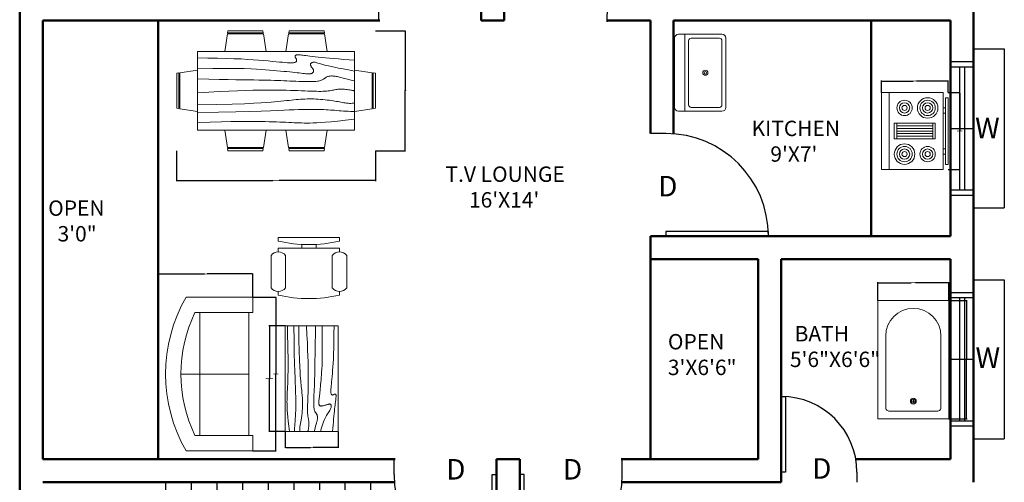
# Model space of a CAD drawing. Units: inches. Extents: x -8 to 1354, y -679 to 94.
# Tile 2 of 6: x 4 to 388, y -429 to -248. Entities that reach past the tile are written whole.
import ezdxf

# ---------------------------------------------------------------- set-up
doc = ezdxf.new("R2010")
doc.units = ezdxf.units.IN
doc.header["$MEASUREMENT"] = 0
for name, color, linetype, lineweight in [('A-ANNO-DIMS', 2, 'Continuous', 18), ('A-ANNO-TEXT', 7, 'Continuous', 25), ('A-AREA-IDEN', 7, 'Continuous', 25), ('A-DOOR', 3, 'Continuous', 25), ('A-FLOR-FIXT', 8, 'Continuous', 18), ('A-FLOR-STRS', 2, 'Continuous', 25), ('A-FURN', 8, 'Continuous', 18), ('A-GLAZ', 4, 'Continuous', 25), ('A-WALL', 1, 'Continuous', 50)]:
    doc.layers.add(name, color=color, linetype=linetype, lineweight=lineweight)
doc.styles.get("Standard").update_dxf_attribs({"font": 'arial.ttf'})
doc.dimstyles.get("Standard").update_dxf_attribs({"dimtxt": 0.18, "dimasz": 0.18, "dimexe": 0.18, "dimexo": 0.0625, "dimgap": 0.09, "dimtad": 0, "dimtih": 1, "dimtoh": 1, "dimdec": 1, "dimzin": 0, "dimdsep": 46, "dimlunit": 4, "dimtxsty": 'Standard', "dimcen": 0.09, "dimclrd": 2, "dimclre": 3, "dimclrt": 6, "dimadec": 0, "dimazin": 0, "dimtfac": 1, "dimtdec": 1, "dimtofl": 0, "dimtmove": 0, "dimatfit": 3, "dimfxl": 1, "dimtfill": 2, "dimtfillclr": 4, "dimtolj": 1, "dimtzin": 0, "dimarcsym": 0})

# ---------------------------------------------------------------- blocks, each defined once
blk = doc.blocks.new('*U5')
for p, q in [((-40, 0), (-40, 6)), ((0, 0), (0, 6))]:
    blk.add_line(p, q)
blk.add_lwpolyline([(0, 0), (0, -40), (-1.75, -40), (-1.75, 0)], close=True)
blk.add_arc((0, 0), 40, 180, 270)
blk = doc.blocks.new('*U4')
for p, q in [((0, 0), (0, -100)), ((750, 0), (750, -100))]:
    blk.add_line(p, q)
blk.add_lwpolyline([(0, 0), (0, 750), (43.75, 750), (43.75, 0)], close=True)
blk.add_arc((0, 0), 750, 0, 90)
blk = doc.blocks.new('*U2')
for p, q in [((0, 0), (0, 6)), ((40, 0), (40, 6))]:
    blk.add_line(p, q)
blk.add_lwpolyline([(0, 0), (0, -40), (1.75, -40), (1.75, 0)], close=True)
blk.add_arc((0, 0), 40, 270, 0)
blk = doc.blocks.new('*U6')
for p, q in [((0, 0), (0, -6)), ((-40, 0), (-40, -6))]:
    blk.add_line(p, q)
blk.add_lwpolyline([(0, 0), (0, 40), (-1.75, 40), (-1.75, 0)], close=True)
blk.add_arc((0, 0), 40, 90, 180)
blk = doc.blocks.new('Chair - Desk')
for p, q in [((-8.5, 0), (-8.5, -1)), ((-8.5, 0), (8.5, 0)), ((8.5, 0), (8.5, -1)), ((-2, -3), (-2, -1.9355)), ((2, -1.9576), (2, -3)), ((-10.5, -5), (-10.5, -14)), ((-8.5, -3), (-8.5, -4)), ((-8.5, -3), (8.5, -3)), ((-6.5, -14), (-6.5, -5)), ((6.5, -5), (6.5, -14)), ((8.5, -3), (8.5, -4)), ((10.5, -14), (10.5, -5)), ((-8.5, -15), (-8.5, -16)), ((8.5, -15), (8.5, -16))]:
    blk.add_line(p, q)
for centre, radius, start, end in [((0, 34.625), 36.625, 256.5803, 283.4197), ((-8.5, -6.5), 2.5, 36.8699, 143.1301), ((8.5, -6.5), 2.5, 36.8699, 143.1301), ((-8.5, -12.5), 2.5, 216.8699, 323.1301), ((0, 19.625), 36.625, 256.5803, 283.4197), ((8.5, -12.5), 2.5, 216.8699, 323.1301)]:
    blk.add_arc(centre, radius, start, end)
blk = doc.blocks.new('Dining Set - 36 x 72 in.')
for p, q in [((-22, 27.5), (-22.1562, 26.50042)), ((-22, 27.5), (-6, 27.5)), ((-5.8437, 26.49966), (-6, 27.5)), ((6, 27.5), (5.8438, 26.50042)), ((6, 27.5), (22, 27.5)), ((22.1563, 26.49966), (22, 27.5)), ((-22.2343, 26.00059), (-23.4847, 17.99762)), ((-22.2304, 26), (-5.7608, 26)), ((-5.8416, 26.5), (-22.1534, 26.5)), ((-4.5152, 17.99762), (-5.7655, 25.99926)), ((5.7657, 26.00059), (4.5153, 17.99762)), ((5.7696, 26), (22.2392, 26)), ((22.1584, 26.5), (5.8466, 26.5)), ((23.4848, 17.99762), (22.2345, 25.99926)), ((36, 18), (-36, 18)), ((-36, 18), (-36, -18)), ((36, -18), (36, 18)), ((-44.0006, 8.23428), (-35.9976, 9.48474)), ((44.0006, 8.23428), (35.9976, 9.48474)), ((-45.5, 8), (-44.5004, 8.15617)), ((-45.5, 8), (-45.5, -8)), ((-44.5, -8.15843), (-44.5, 8.15338)), ((-44, 8.23041), (-44, -8.23915)), ((44, 8.23041), (44, -8.23915)), ((44.5, -8.15843), (44.5, 8.15338)), ((45.5, 8), (44.5005, 8.15617)), ((45.5, 8), (45.5, -8)), ((-44.4997, -8.15631), (-45.5, -8)), ((-35.9976, -9.48476), (-43.9993, -8.2345)), ((35.9976, -9.48476), (43.9993, -8.2345)), ((44.4997, -8.15631), (45.5, -8)), ((-36, -18), (36, -18)), ((-22.2343, -26.0006), (-23.4847, -17.99762)), ((-4.5152, -17.99762), (-5.7655, -25.99928)), ((5.7657, -26.0006), (4.5153, -17.99762)), ((23.4848, -17.99762), (22.2345, -25.99928)), ((-22.2304, -26), (-5.7608, -26)), ((-22, -27.5), (-22.1562, -26.50044)), ((-5.8416, -26.5), (-22.1534, -26.5)), ((-5.8437, -26.49967), (-6, -27.5)), ((5.7696, -26), (22.2392, -26)), ((6, -27.5), (5.8438, -26.50044)), ((22.1584, -26.5), (5.8466, -26.5)), ((22.1563, -26.49967), (22, -27.5)), ((-22, -27.5), (-6, -27.5)), ((6, -27.5), (22, -27.5))]:
    blk.add_line(p, q)
for points in [[(-36, 15), (-31.1772, 14.97754), (-26.8079, 14.91406), (-22.8538, 14.81543), (-19.276, 14.6875), (-16.0362, 14.53613), (-13.0957, 14.36718), (-10.4159, 14.18652), (-7.9583, 14), (-5.6904, 13.81315), (-3.6035, 13.63021), (-1.6954, 13.45508), (0.0365, 13.29166), (1.5945, 13.14388), (2.9811, 13.01562), (4.1988, 12.9108), (5.25, 12.83333), (6.1393, 12.78613), (6.8802, 12.76823), (7.4883, 12.77767), (7.9792, 12.8125), (8.3685, 12.87077), (8.6719, 12.95052), (8.9049, 13.0498), (9.0833, 13.16666), (9.2205, 13.29899), (9.3216, 13.44401), (9.3895, 13.59879), (9.4271, 13.76041), (9.4373, 13.92594), (9.4232, 14.09245), (9.3875, 14.257), (9.3333, 14.41666), (9.2638, 14.56917), (9.1836, 14.71484), (9.0975, 14.85465), (9.0104, 14.98958), (8.9272, 15.1206), (8.8529, 15.2487), (8.7922, 15.37483), (8.75, 15.5), (8.7305, 15.62467), (8.7344, 15.74739), (8.7617, 15.86621), (8.8125, 15.97916), (8.8867, 16.08431), (8.9844, 16.17968), (9.1055, 16.26334), (9.25, 16.33333), (9.4189, 16.38802), (9.6172, 16.42708), (9.8506, 16.45052), (10.125, 16.45833), (10.4463, 16.45052), (10.8203, 16.42708), (11.2529, 16.38802), (11.75, 16.33333), (12.3184, 16.26318), (12.9694, 16.17838), (13.7151, 16.07991), (14.5677, 15.96875), (15.5395, 15.84586), (16.6426, 15.71224), (17.8893, 15.56884), (19.2917, 15.41666), (20.859, 15.25667), (22.5879, 15.08984), (24.4721, 14.91715), (26.5052, 14.73958), (28.6809, 14.5581), (30.9929, 14.3737), (33.4347, 14.18733), (36, 14)], [(-36, 10), (-28.9766, 10.14274), (-23.1725, 10.20442), (-18.4241, 10.19775), (-14.5677, 10.13541), (-11.4399, 10.03011), (-8.877, 9.89453), (-6.7154, 9.74137), (-4.7917, 9.58333), (-2.9698, 9.43082), (-1.2246, 9.28515), (0.4415, 9.14534), (2.026, 9.01041), (3.5266, 8.87939), (4.9408, 8.7513), (6.266, 8.62516), (7.5, 8.5), (8.6411, 8.37549), (9.6914, 8.2539), (10.6538, 8.13818), (11.5312, 8.03125), (12.3267, 7.93603), (13.043, 7.85547), (13.6831, 7.79248), (14.25, 7.75), (14.7471, 7.7303), (15.1797, 7.73307), (15.5537, 7.75732), (15.875, 7.80208), (16.1494, 7.86637), (16.3828, 7.94922), (16.5811, 8.04964), (16.75, 8.16666), (16.8944, 8.29915), (17.0143, 8.44531), (17.1089, 8.60319), (17.1771, 8.77083), (17.218, 8.94629), (17.2305, 9.1276), (17.2137, 9.31282), (17.1667, 9.5), (17.0895, 9.6875), (16.987, 9.875), (16.8649, 10.0625), (16.7292, 10.25), (16.5856, 10.4375), (16.4401, 10.625), (16.2985, 10.8125), (16.1667, 11), (16.05, 11.18733), (15.9518, 11.3737), (15.8752, 11.5581), (15.8229, 11.73958), (15.798, 11.91715), (15.8034, 12.08984), (15.842, 12.25667), (15.9167, 12.41666), (16.0295, 12.56836), (16.1784, 12.70833), (16.3605, 12.83268), (16.5729, 12.9375), (16.8127, 13.01888), (17.0768, 13.07291), (17.3625, 13.0957), (17.6667, 13.08333), (17.9894, 13.03312), (18.3418, 12.94726), (18.7382, 12.82918), (19.1927, 12.68229), (19.7195, 12.51001), (20.3327, 12.31575), (21.0465, 12.10294), (21.875, 11.875), (22.8357, 11.63354), (23.959, 11.37304), (25.2786, 11.08618), (26.8282, 10.76562), (28.6414, 10.40405), (30.752, 9.99414), (33.1936, 9.52856), (36, 9)], [(-36, 5.5), (-30.7157, 5.3348), (-26.069, 5.20963), (-21.9946, 5.11767), (-18.4271, 5.05208), (-15.3009, 5.00602), (-12.5508, 4.97265), (-10.1112, 4.94515), (-7.9167, 4.91666), (-5.909, 4.88167), (-4.0586, 4.83984), (-2.3429, 4.79215), (-0.7396, 4.73958), (0.7739, 4.6831), (2.22, 4.6237), (3.6213, 4.56233), (5, 4.5), (6.373, 4.43782), (7.7344, 4.3776), (9.0723, 4.32129), (10.375, 4.27083), (11.6309, 4.22819), (12.8281, 4.19531), (13.9551, 4.17415), (15, 4.16666), (15.954, 4.17448), (16.819, 4.19791), (17.6001, 4.23698), (18.3021, 4.29166), (18.9299, 4.36198), (19.4883, 4.44791), (19.9823, 4.54948), (20.4167, 4.66666), (20.7969, 4.79899), (21.1302, 4.94401), (21.4245, 5.09879), (21.6875, 5.26041), (21.9271, 5.42594), (22.1511, 5.59245), (22.3672, 5.757), (22.5834, 5.91666), (22.8065, 6.06868), (23.0404, 6.21093), (23.2879, 6.34147), (23.5521, 6.45833), (23.8358, 6.55957), (24.142, 6.64323), (24.4735, 6.70735), (24.8334, 6.75), (25.2235, 6.76969), (25.642, 6.76692), (26.0858, 6.74267), (26.5521, 6.69791), (27.0379, 6.63362), (27.5404, 6.55078), (28.0565, 6.45036), (28.5834, 6.33333), (29.1242, 6.19987), (29.7071, 6.04687), (30.3661, 5.87044), (31.1354, 5.66666), (32.0493, 5.43164), (33.142, 5.16146), (34.4475, 4.85221), (36, 4.5)], [(-36, -1), (-30.7915, -0.6591), (-26.0195, -0.38216), (-21.6519, -0.16284), (-17.6563, 0.00521), (-14.0005, 0.12833), (-10.6523, 0.21289), (-7.5796, 0.26522), (-4.75, 0.29166), (-2.134, 0.29793), (0.2878, 0.28711), (2.5317, 0.26163), (4.6146, 0.22396), (6.5529, 0.17651), (8.3633, 0.12174), (10.0623, 0.06209), (11.6667, 0), (13.1899, -0.06201), (14.6341, -0.1211), (15.9982, -0.17432), (17.2813, -0.21875), (18.4823, -0.25147), (19.6003, -0.26953), (20.6343, -0.27002), (21.5834, -0.25), (22.4481, -0.20768), (23.2357, -0.14584), (23.9549, -0.06836), (24.6146, 0.02083), (25.2235, 0.11784), (25.7904, 0.21875), (26.3241, 0.31966), (26.8334, 0.41666), (27.3265, 0.50618), (27.8099, 0.58593), (28.2894, 0.65397), (28.7709, 0.70833), (29.2601, 0.74707), (29.763, 0.76823), (30.2855, 0.76985), (30.8334, 0.75), (31.4088, 0.70784), (31.9994, 0.64713), (32.589, 0.57275), (33.1615, 0.48958), (33.7008, 0.4025), (34.1908, 0.3164), (34.6153, 0.23616), (34.9584, 0.16666), (35.2099, 0.11165), (35.3848, 0.07031), (35.504, 0.04069), (35.5886, 0.02083), (35.6594, 0.00879), (35.7377, 0.0026), (35.8442, 0.00032), (36, 0)], [(-36, -6.5), (-27.1843, -6.31267), (-20.084, -6.1263), (-14.469, -5.9419), (-10.1094, -5.76042), (-6.7752, -5.58285), (-4.2363, -5.41016), (-2.2629, -5.24333), (-0.625, -5.08334), (0.8708, -4.93099), (2.2715, -4.78646), (3.5872, -4.64974), (4.8281, -4.52084), (6.0046, -4.39974), (7.127, -4.28646), (8.2053, -4.18099), (9.25, -4.08334), (10.2705, -3.99382), (11.2734, -3.91407), (12.2647, -3.84603), (13.25, -3.79167), (14.2354, -3.75293), (15.2266, -3.73177), (16.2295, -3.73015), (17.25, -3.75), (18.2912, -3.79248), (19.3451, -3.85547), (20.4009, -3.93604), (21.4479, -4.03125), (22.4754, -4.13819), (23.4727, -4.25391), (24.4289, -4.37549), (25.3334, -4.5), (26.1785, -4.62492), (26.9694, -4.74935), (27.7145, -4.87281), (28.4219, -4.99479), (29.1, -5.11483), (29.7572, -5.23242), (30.4016, -5.34709), (31.0417, -5.45834), (31.6837, -5.56437), (32.3262, -5.65821), (32.9658, -5.73153), (33.599, -5.77604), (34.2224, -5.78345), (34.8327, -5.74545), (35.4264, -5.65373), (36, -5.5)], [(-36, -10), (-26.4022, -9.81299), (-18.4675, -9.62891), (-11.9839, -9.45069), (-6.7396, -9.28125), (-2.5226, -9.12354), (0.8789, -8.98047), (3.6769, -8.85498), (6.0833, -8.75), (8.2767, -8.66765), (10.3021, -8.60677), (12.1712, -8.56543), (13.8958, -8.54167), (15.4876, -8.53353), (16.9583, -8.53907), (18.3197, -8.55632), (19.5834, -8.58334), (20.7616, -8.61841), (21.8685, -8.66081), (22.9188, -8.71004), (23.9271, -8.76563), (24.9081, -8.82707), (25.8763, -8.89388), (26.8465, -8.96558), (27.8334, -9.04167), (28.8474, -9.12118), (29.8828, -9.20117), (30.93, -9.27824), (31.9792, -9.34896), (33.0205, -9.40991), (34.0443, -9.45768), (35.0407, -9.48885), (36, -9.5)], [(-36, -14.5), (-30.0881, -14.33513), (-25.0332, -14.21224), (-20.7312, -14.12647), (-17.0781, -14.07292), (-13.97, -14.04671), (-11.3027, -14.04297), (-8.9724, -14.05681), (-6.875, -14.08334), (-4.9224, -14.11833), (-3.0905, -14.16016), (-1.3709, -14.20785), (0.2448, -14.26042), (1.7647, -14.3169), (3.1973, -14.3763), (4.5507, -14.43767), (5.8333, -14.5), (7.0554, -14.5621), (8.235, -14.62175), (9.3922, -14.67652), (10.5469, -14.72396), (11.7192, -14.76164), (12.929, -14.78711), (14.1965, -14.79794), (15.5417, -14.79167), (16.9933, -14.76424), (18.6152, -14.70508), (20.4804, -14.60197), (22.6615, -14.44271), (25.2312, -14.21509), (28.2624, -13.9069), (31.8277, -13.50594), (36, -13)]]:
    blk.add_lwpolyline(points)
blk = doc.blocks.new('Sofa - Roundback Loveseat 5 ft.')
for p, q in [((0, -32.44198), (0, -5.99998)), ((-24, -33.99998), (-24, -11.46958)), ((24.00004, -33.99998), (24.00004, -11.46958)), ((-23.9998, -13.38178), (23.99986, -13.38178)), ((-24, -32.44198), (24.00004, -32.44198))]:
    blk.add_line(p, q)
for points in [[(-24, -33.99998), (-30, -33.99998), (-30, -7.99998)], [(30.00004, -7.99998), (30.00004, -33.99998), (24.00004, -33.99998)]]:
    blk.add_lwpolyline(points)
for centre, radius, start, end in [((0, -60.24998), 60.24998, 60.13715, 119.8628), ((0, -61.38438), 55.38444, 64.32083, 115.6792)]:
    blk.add_arc(centre, radius, start, end)
blk = doc.blocks.new('Table - Rectangular Woodgrain 60 x 30 in.')
for p, q in [((0, 0), (0, -30)), ((60, 0), (0, 0)), ((60, -30), (60, 0)), ((0, -30), (60, -30))]:
    blk.add_line(p, q)
for points in [[(0, -2.4), (4.8155, -2.418), (9.0302, -2.4688), (12.709, -2.5477), (15.9167, -2.65), (18.7181, -2.7711), (21.1781, -2.9063), (23.3616, -3.0508), (25.3333, -3.2), (27.1477, -3.3495), (28.8172, -3.4958), (30.3437, -3.636), (31.7291, -3.7667), (32.9756, -3.8849), (34.0849, -3.9875), (35.059, -4.0714), (35.9, -4.1334), (36.6114, -4.1711), (37.2041, -4.1854), (37.6906, -4.1779), (38.0833, -4.15), (38.3948, -4.1034), (38.6375, -4.0396), (38.8239, -3.9602), (38.9666, -3.8667), (39.0764, -3.7608), (39.1573, -3.6448), (39.2116, -3.521), (39.2416, -3.3917), (39.2498, -3.2593), (39.2385, -3.1261), (39.21, -2.9944), (39.1666, -2.8667), (39.111, -2.7447), (39.0468, -2.6281), (38.978, -2.5163), (38.9083, -2.4083), (38.8418, -2.3035), (38.7823, -2.201), (38.7337, -2.1001), (38.7, -2), (38.6844, -1.9003), (38.6875, -1.8021), (38.7094, -1.707), (38.75, -1.6167), (38.8094, -1.5326), (38.8875, -1.4563), (38.9844, -1.3893), (39.1, -1.3333), (39.2351, -1.2896), (39.3937, -1.2583), (39.5804, -1.2396), (39.8, -1.2333), (40.057, -1.2396), (40.3562, -1.2583), (40.7023, -1.2896), (41.1, -1.3333), (41.5547, -1.3895), (42.0755, -1.4573), (42.6721, -1.5361), (43.3542, -1.625), (44.1316, -1.7233), (45.014, -1.8302), (46.0114, -1.9449), (47.1333, -2.0667), (48.3862, -2.1947), (49.7625, -2.3281), (51.2513, -2.4663), (52.8416, -2.6083), (54.5226, -2.7535), (56.2833, -2.9011), (58.1127, -3.0501), (60, -3.2)], [(0, -9.2), (6.5759, -9.0858), (11.9385, -9.0365), (16.2527, -9.0418), (19.6833, -9.0917), (22.3952, -9.1759), (24.5531, -9.2844), (26.322, -9.4069), (27.8666, -9.5333), (29.3241, -9.6553), (30.7203, -9.7719), (32.0532, -9.8837), (33.3208, -9.9917), (34.5213, -10.0965), (35.6526, -10.199), (36.7128, -10.2999), (37.7, -10.4), (38.6129, -10.4996), (39.4531, -10.5969), (40.223, -10.6895), (40.925, -10.775), (41.5613, -10.8512), (42.1344, -10.9156), (42.6465, -10.966), (43.1, -11), (43.4976, -11.0158), (43.8437, -11.0136), (44.143, -10.9942), (44.4, -10.9583), (44.6195, -10.9069), (44.8062, -10.8406), (44.9648, -10.7603), (45.1, -10.6667), (45.2155, -10.5598), (45.3114, -10.4365), (45.3871, -10.2929), (45.4416, -10.125), (45.4743, -9.929), (45.4844, -9.7011), (45.4709, -9.4371), (45.4333, -9.1333), (45.3716, -8.7883), (45.2896, -8.4104), (45.1919, -8.0107), (45.0833, -7.6), (44.9685, -7.1893), (44.8521, -6.7896), (44.7388, -6.4117), (44.6333, -6.0667), (44.54, -5.7628), (44.4614, -5.4979), (44.4001, -5.2675), (44.3583, -5.0667), (44.3384, -4.8909), (44.3427, -4.7354), (44.3736, -4.5956), (44.4333, -4.4667), (44.5236, -4.3453), (44.6427, -4.2333), (44.7884, -4.1339), (44.9583, -4.05), (45.1501, -3.9849), (45.3614, -3.9417), (45.59, -3.9234), (45.8333, -3.9333), (46.0915, -3.9749), (46.3734, -4.0531), (46.6906, -4.1736), (47.0542, -4.3417), (47.4756, -4.5629), (47.9661, -4.8427), (48.5372, -5.1866), (49.2, -5.6), (49.9676, -6.0844), (50.8594, -6.625), (51.8965, -7.2031), (53.1, -7.8), (54.491, -8.3969), (56.0906, -8.975), (57.9199, -9.5156), (60, -10)], [(0, -12.8), (5.1847, -12.9322), (9.6213, -13.0323), (13.3963, -13.1059), (16.5958, -13.1583), (19.3063, -13.1952), (21.614, -13.2219), (23.6054, -13.2439), (25.3666, -13.2667), (26.9728, -13.2947), (28.4531, -13.3281), (29.8256, -13.3663), (31.1083, -13.4083), (32.3191, -13.4535), (33.476, -13.501), (34.597, -13.5501), (35.7, -13.6), (36.7984, -13.6497), (37.8875, -13.6979), (38.9578, -13.743), (40, -13.7833), (41.0047, -13.8174), (41.9625, -13.8438), (42.864, -13.8607), (43.7, -13.8667), (44.4631, -13.8604), (45.1552, -13.8417), (45.7801, -13.8104), (46.3416, -13.7667), (46.8439, -13.7104), (47.2906, -13.6417), (47.6858, -13.5604), (48.0333, -13.4667), (48.3375, -13.3608), (48.6042, -13.2448), (48.8396, -13.121), (49.05, -12.9917), (49.2417, -12.8593), (49.4208, -12.7261), (49.5937, -12.5944), (49.7667, -12.4667), (49.9452, -12.3451), (50.1323, -12.2313), (50.3303, -12.1268), (50.5416, -12.0333), (50.7686, -11.9524), (51.0135, -11.8854), (51.2788, -11.8341), (51.5666, -11.8), (51.8785, -11.7843), (52.2116, -11.7865), (52.562, -11.8059), (52.926, -11.8417), (53.2998, -11.8931), (53.6795, -11.9594), (54.0614, -12.0397), (54.4416, -12.1333), (54.8223, -12.2401), (55.2293, -12.3625), (55.6942, -12.5037), (56.2489, -12.6667), (56.9251, -12.8547), (57.7545, -13.0708), (58.7689, -13.3182), (60, -13.6)], [(0, -18), (5.124, -17.7273), (9.6609, -17.5057), (13.6705, -17.3303), (17.2125, -17.1958), (20.3467, -17.0973), (23.1328, -17.0297), (25.6307, -16.9878), (27.9, -16.9667), (29.9928, -16.9617), (31.9302, -16.9703), (33.7254, -16.9907), (35.3917, -17.0208), (36.9423, -17.0588), (38.3906, -17.1026), (39.7499, -17.1503), (41.0333, -17.2), (42.2519, -17.2496), (43.4073, -17.2969), (44.4986, -17.3395), (45.525, -17.375), (46.4858, -17.4012), (47.3802, -17.4156), (48.2074, -17.416), (48.9667, -17.4), (49.6583, -17.3662), (50.2872, -17.3167), (50.8595, -17.2547), (51.3812, -17.1833), (51.8584, -17.1057), (52.2971, -17.025), (52.7034, -16.9443), (53.0833, -16.8667), (53.443, -16.7951), (53.789, -16.7313), (54.128, -16.6768), (54.4666, -16.6334), (54.8115, -16.6024), (55.1693, -16.5854), (55.5465, -16.5841), (55.95, -16.6), (56.3828, -16.6337), (56.8346, -16.6823), (57.2915, -16.7418), (57.7396, -16.8084), (58.165, -16.878), (58.5539, -16.9469), (58.8924, -17.0111), (59.1666, -17.0667), (59.3679, -17.1107), (59.5078, -17.1438), (59.6032, -17.1675), (59.6708, -17.1833), (59.7275, -17.193), (59.7901, -17.1979), (59.8753, -17.1998), (60, -17.2)], [(0, -22.4), (8.0098, -22.2501), (14.4094, -22.1011), (19.4168, -21.9535), (23.25, -21.8083), (26.1269, -21.6663), (28.2656, -21.5281), (29.884, -21.3947), (31.2, -21.2667), (32.3967, -21.1448), (33.5172, -21.0292), (34.5697, -20.9198), (35.5625, -20.8167), (36.5037, -20.7198), (37.4015, -20.6292), (38.2642, -20.5448), (39.1, -20.4667), (39.9164, -20.3951), (40.7187, -20.3313), (41.5117, -20.2768), (42.3, -20.2333), (43.0883, -20.2024), (43.8812, -20.1854), (44.6836, -20.1841), (45.5, -20.2), (46.3328, -20.234), (47.1747, -20.2844), (48.0163, -20.3488), (48.8479, -20.425), (49.66, -20.5106), (50.4429, -20.6031), (51.1872, -20.7004), (51.8833, -20.8), (52.5246, -20.8999), (53.1166, -20.9995), (53.6681, -21.0983), (54.1875, -21.1958), (54.6834, -21.2919), (55.1646, -21.3859), (55.6394, -21.4777), (56.1167, -21.5667), (56.6028, -21.6515), (57.0961, -21.7266), (57.5929, -21.7852), (58.0896, -21.8208), (58.5823, -21.8268), (59.0674, -21.7964), (59.5412, -21.723), (60, -21.6)], [(0, -25.2), (8.6355, -25.0504), (15.7026, -24.9031), (21.4049, -24.7606), (25.9458, -24.625), (29.529, -24.4988), (32.3578, -24.3844), (34.6359, -24.284), (36.5667, -24.2), (38.3213, -24.1341), (39.9417, -24.0854), (41.437, -24.0523), (42.8167, -24.0333), (44.0901, -24.0268), (45.2667, -24.0313), (46.3557, -24.0451), (47.3667, -24.0667), (48.309, -24.0947), (49.1928, -24.1287), (50.0284, -24.168), (50.826, -24.2125), (51.5959, -24.2617), (52.3483, -24.3151), (53.0935, -24.3725), (53.8417, -24.4334), (54.6009, -24.497), (55.3699, -24.561), (56.1454, -24.6226), (56.9239, -24.6792), (57.7021, -24.7279), (58.4764, -24.7662), (59.2435, -24.7911), (60, -24.8)], [(0, -28.8), (5.6867, -28.6681), (10.45, -28.5698), (14.407, -28.5012), (17.675, -28.4584), (20.3711, -28.4374), (22.6125, -28.4344), (24.5164, -28.4455), (26.2, -28.4667), (27.762, -28.4947), (29.2276, -28.5281), (30.6033, -28.5663), (31.8958, -28.6084), (33.1118, -28.6535), (34.2578, -28.7011), (35.3405, -28.7501), (36.3666, -28.8), (37.3443, -28.8497), (38.288, -28.8974), (39.2137, -28.9412), (40.1375, -28.9792), (41.0753, -29.0093), (42.0432, -29.0297), (43.0572, -29.0384), (44.1333, -29.0333), (45.2936, -29.0114), (46.5843, -28.9641), (48.0579, -28.8816), (49.7666, -28.7542), (51.7629, -28.5721), (54.0989, -28.3255), (56.8272, -28.0048), (60, -27.6)]]:
    blk.add_lwpolyline(points)
blk = doc.blocks.new('Bath Tub - 26 x 60 in.')
for p, q in [((8, -18), (10, -18)), ((9, -17), (9, -19))]:
    blk.add_line(p, q)
blk.add_lwpolyline([(0, -36), (0, 0), (60, 0), (60, -36)], close=True)
for points in [[(6, -4), (42, -4)], [(4, -30), (4, -6)], [(42, -32), (6, -32)]]:
    blk.add_lwpolyline(points)
for radius in [1.5, 1]:
    blk.add_circle((9, -18), radius)
for centre, radius, start, end in [((5.75, -5.75), 1.77, 81.8699, 188.1301), ((42, -18), 14, 270, 90), ((5.75, -30.25), 1.77, 171.8699, 278.1301)]:
    blk.add_arc(centre, radius, start, end)
blk = doc.blocks.new('Sink-single - 30 in top')
blk.add_line((-15, -3.999996), (15, -3.999996))
for points in [[(-13.5, 0), (13.5, 0)], [(-15, -18.499996), (-15, -1.5)], [(15, -1.5), (15, -18.499996)], [(-13.5, -17.499996), (-13.5, -6.499996)], [(-12.5, -5.499996), (12.5, -5.499996)], [(13.5, -6.499996), (13.5, -17.499996)], [(12.5, -18.499996), (-12.5, -18.499996)], [(13.5, -19.999996), (-13.5, -19.999996)]]:
    blk.add_lwpolyline(points)
for radius in [1, 0.5]:
    blk.add_circle((0, -11.999996), radius)
for centre, radius, start, end in [((-13.5, -1.5), 1.5, 90, 180), ((13.5, -1.5), 1.5, 0, 90), ((-12.5, -6.499996), 1, 90, 180), ((12.5, -6.499996), 1, 0, 90), ((-13.5, -18.499996), 1.5, 180, 270), ((-12.5, -17.499996), 1, 180, 270), ((12.5, -17.499996), 1, 270, 0), ((13.5, -18.499996), 1.5, 270, 0)]:
    blk.add_arc(centre, radius, start, end)
blk = doc.blocks.new('Range-Oven - 30 in top')
for p, q in [((0, -3), (30, -3)), ((12, -6), (18, -6)), ((13, -20), (13, -6)), ((14, -6), (14, -20)), ((15, -20), (15, -6)), ((16, -6), (16, -20)), ((17, -20), (17, -6)), ((18, -20), (12, -20)), ((6, -24), (6, -25)), ((8, -25), (8, -24)), ((22, -25), (22, -24)), ((24, -24), (24, -25))]:
    blk.add_line(p, q)
for points in [[(0, -24), (0, 0), (30, 0), (30, -24)], [(12, -21), (12, -5), (18, -5), (18, -21)], [(2, -26), (2, -25), (28, -25), (28, -26)]]:
    blk.add_lwpolyline(points, close=True)
for centre, radius in [((6, -9), 4), ((6, -9), 3), ((6, -9), 2), ((24, -9), 3), ((24, -9), 2), ((6, -9), 1), ((24, -9), 1), ((6, -18), 3), ((24, -18), 4), ((24, -18), 3), ((6, -18), 2), ((6, -18), 1), ((24, -18), 2), ((24, -18), 1)]:
    blk.add_circle(centre, radius)
blk = doc.blocks.new('WIN-W')
at = {"ltscale": 2}
for p, q in [((12, 62), (0, 62)), ((0, 0), (0, 62)), ((12, 57), (12, 62)), ((12, 5), (12, 0)), ((12, 0), (0, 0))]:
    blk.add_line(p, q, dxfattribs=at)
for p, q in [((21, 57), (12, 57)), ((21, 5), (12, 5))]:
    blk.add_line(p, q)
blk = doc.blocks.new('*D99')
at = {"layer": 'A-ANNO-DIMS', "color": 3, "lineweight": -2, "transparency": 16777216}
for p, q in [((107.68, -367.77), (101.37, -367.77)), ((107.68, -409.08), (101.37, -409.08))]:
    blk.add_line(p, q, dxfattribs=at)
at = {"layer": 'A-ANNO-DIMS', "color": 2, "lineweight": -2, "transparency": 16777216}
for p, q in [((101.55, -367.95), (101.55, -388.24)), ((101.55, -408.9), (101.55, -388.61))]:
    blk.add_line(p, q, dxfattribs=at)
at = {"layer": 'A-ANNO-DIMS', "color": 2, "transparency": 16777216}
for points in [[(101.52, -367.95), (101.58, -367.95), (101.55, -367.77)], [(101.52, -408.9), (101.58, -408.9), (101.55, -409.08)]]:
    blk.add_solid(points, dxfattribs=at)
at = {"layer": 'Defpoints', "color": 0, "transparency": 16777216}
for p in [(107.74, -367.77), (101.55, -409.08), (107.74, -409.08)]:
    blk.add_point(p, dxfattribs=at)
at = {"layer": 'A-ANNO-DIMS', "color": 6, "transparency": 16777216, "insert": (101.55, -388.42), "char_height": 0.18, "attachment_point": 5, "bg_fill": 1, "box_fill_scale": 1.25, "bg_fill_color": 4, "bg_fill_transparency": 0}
blk.add_mtext('\\A1;COFFEE TABLE 3\'-5 1/2"', dxfattribs=at)
blk = doc.blocks.new('*D100')
at = {"layer": 'A-ANNO-DIMS', "color": 3, "lineweight": -2, "transparency": 16777216}
for p, q in [((107.74, -409.14), (107.74, -415.45)), ((128.4, -409.14), (128.4, -415.45))]:
    blk.add_line(p, q, dxfattribs=at)
at = {"layer": 'A-ANNO-DIMS', "color": 2, "lineweight": -2, "transparency": 16777216}
for p, q in [((107.92, -415.27), (117.54, -415.27)), ((128.22, -415.27), (118.6, -415.27))]:
    blk.add_line(p, q, dxfattribs=at)
at = {"layer": 'A-ANNO-DIMS', "color": 2, "transparency": 16777216}
for points in [[(107.92, -415.24), (107.92, -415.3), (107.74, -415.27)], [(128.22, -415.24), (128.22, -415.3), (128.4, -415.27)]]:
    blk.add_solid(points, dxfattribs=at)
at = {"layer": 'Defpoints', "color": 0, "transparency": 16777216}
for p in [(107.74, -409.08), (128.4, -409.08), (128.4, -415.27)]:
    blk.add_point(p, dxfattribs=at)
at = {"layer": 'A-ANNO-DIMS', "color": 6, "transparency": 16777216, "insert": (118.07, -415.27), "char_height": 0.18, "attachment_point": 5, "bg_fill": 1, "box_fill_scale": 1.25, "bg_fill_color": 4, "bg_fill_transparency": 0}
blk.add_mtext('\\A1;1\'-8 1/2"', dxfattribs=at)
blk = doc.blocks.new('*D103')
at = {"layer": 'A-ANNO-DIMS', "color": 3, "lineweight": -2, "transparency": 16777216}
for p, q in [((65.38, -299.65), (65.38, -311.39)), ((142.87, -299.65), (142.87, -311.39))]:
    blk.add_line(p, q, dxfattribs=at)
at = {"layer": 'A-ANNO-DIMS', "color": 2, "lineweight": -2, "transparency": 16777216}
for p, q in [((65.56, -311.21), (102.84, -311.21)), ((142.69, -311.21), (105.42, -311.21))]:
    blk.add_line(p, q, dxfattribs=at)
at = {"layer": 'A-ANNO-DIMS', "color": 2, "transparency": 16777216}
for points in [[(65.56, -311.18), (65.56, -311.24), (65.38, -311.21)], [(142.69, -311.18), (142.69, -311.24), (142.87, -311.21)]]:
    blk.add_solid(points, dxfattribs=at)
at = {"layer": 'Defpoints', "color": 0, "transparency": 16777216}
for p in [(65.38, -299.58), (142.87, -299.58), (142.87, -311.21)]:
    blk.add_point(p, dxfattribs=at)
at = {"layer": 'A-ANNO-DIMS', "color": 6, "transparency": 16777216, "insert": (104.13, -311.21), "char_height": 0.18, "attachment_point": 5, "bg_fill": 1, "box_fill_scale": 1.25, "bg_fill_color": 4, "bg_fill_transparency": 0}
blk.add_mtext('\\A1;DINING SET 6\'-5 1/2"', dxfattribs=at)
blk = doc.blocks.new('*D104')
at = {"layer": 'A-ANNO-DIMS', "color": 3, "lineweight": -2, "transparency": 16777216}
for p, q in [((142.94, -252.75), (154.68, -252.75)), ((142.94, -299.58), (154.68, -299.58))]:
    blk.add_line(p, q, dxfattribs=at)
at = {"layer": 'A-ANNO-DIMS', "color": 2, "lineweight": -2, "transparency": 16777216}
for p, q in [((154.5, -252.93), (154.5, -275.98)), ((154.5, -299.4), (154.5, -276.35))]:
    blk.add_line(p, q, dxfattribs=at)
at = {"layer": 'A-ANNO-DIMS', "color": 2, "transparency": 16777216}
for points in [[(154.47, -252.93), (154.53, -252.93), (154.5, -252.75)], [(154.47, -299.4), (154.53, -299.4), (154.5, -299.58)]]:
    blk.add_solid(points, dxfattribs=at)
at = {"layer": 'Defpoints', "color": 0, "transparency": 16777216}
for p in [(142.87, -252.75), (154.5, -252.75), (142.87, -299.58)]:
    blk.add_point(p, dxfattribs=at)
at = {"layer": 'A-ANNO-DIMS', "color": 6, "transparency": 16777216, "insert": (154.5, -276.17), "char_height": 0.18, "attachment_point": 5, "bg_fill": 1, "box_fill_scale": 1.25, "bg_fill_color": 4, "bg_fill_transparency": 0}
blk.add_mtext('\\A1;3\'-11"', dxfattribs=at)
blk = doc.blocks.new('*D107')
at = {"layer": 'A-ANNO-DIMS', "color": 3, "lineweight": -2, "transparency": 16777216}
for p, q in [((366.59, -357.95), (373.64, -357.95)), ((366.59, -404.12), (373.64, -404.12))]:
    blk.add_line(p, q, dxfattribs=at)
at = {"layer": 'A-ANNO-DIMS', "color": 2, "lineweight": -2, "transparency": 16777216}
for p, q in [((373.46, -358.13), (373.46, -380.85)), ((373.46, -403.94), (373.46, -381.22))]:
    blk.add_line(p, q, dxfattribs=at)
at = {"layer": 'A-ANNO-DIMS', "color": 2, "transparency": 16777216}
for points in [[(373.43, -358.13), (373.49, -358.13), (373.46, -357.95)], [(373.43, -403.94), (373.49, -403.94), (373.46, -404.12)]]:
    blk.add_solid(points, dxfattribs=at)
at = {"layer": 'Defpoints', "color": 0, "transparency": 16777216}
for p in [(366.53, -357.95), (373.46, -357.95), (366.53, -404.12)]:
    blk.add_point(p, dxfattribs=at)
at = {"layer": 'A-ANNO-DIMS', "color": 6, "transparency": 16777216, "insert": (373.46, -381.04), "char_height": 0.18, "attachment_point": 5, "bg_fill": 1, "box_fill_scale": 1.25, "bg_fill_color": 4, "bg_fill_transparency": 0}
blk.add_mtext('\\A1;BATH TUB 3\'-10" TYP.', dxfattribs=at)
blk = doc.blocks.new('*D108')
at = {"layer": 'A-ANNO-DIMS', "color": 3, "lineweight": -2, "transparency": 16777216}
for p, q in [((338.84, -357.89), (338.84, -350.85)), ((366.53, -357.89), (366.53, -350.85))]:
    blk.add_line(p, q, dxfattribs=at)
at = {"layer": 'A-ANNO-DIMS', "color": 2, "lineweight": -2, "transparency": 16777216}
for p, q in [((339.02, -351.03), (351.83, -351.03)), ((366.35, -351.03), (353.53, -351.03))]:
    blk.add_line(p, q, dxfattribs=at)
at = {"layer": 'A-ANNO-DIMS', "color": 2, "transparency": 16777216}
for points in [[(339.02, -351), (339.02, -351.06), (338.84, -351.03)], [(366.35, -351), (366.35, -351.06), (366.53, -351.03)]]:
    blk.add_solid(points, dxfattribs=at)
at = {"layer": 'Defpoints', "color": 0, "transparency": 16777216}
for p in [(338.84, -351.03), (338.84, -357.95), (366.53, -357.95)]:
    blk.add_point(p, dxfattribs=at)
at = {"layer": 'A-ANNO-DIMS', "color": 6, "transparency": 16777216, "insert": (352.68, -351.03), "char_height": 0.18, "attachment_point": 5, "bg_fill": 1, "box_fill_scale": 1.25, "bg_fill_color": 4, "bg_fill_transparency": 0}
blk.add_mtext('\\A1;2\'-3 1/2" TYP.', dxfattribs=at)
blk = doc.blocks.new('*D111')
at = {"layer": 'A-ANNO-DIMS', "color": 3, "lineweight": -2, "transparency": 16777216}
for p, q in [((366.32, -276.87), (370.94, -276.87)), ((366.32, -306.87), (370.94, -306.87))]:
    blk.add_line(p, q, dxfattribs=at)
at = {"layer": 'A-ANNO-DIMS', "color": 2, "lineweight": -2, "transparency": 16777216}
for p, q in [((370.76, -277.05), (370.76, -291.69)), ((370.76, -306.69), (370.76, -292.06))]:
    blk.add_line(p, q, dxfattribs=at)
at = {"layer": 'A-ANNO-DIMS', "color": 2, "transparency": 16777216}
for points in [[(370.73, -277.05), (370.79, -277.05), (370.76, -276.87)], [(370.73, -306.69), (370.79, -306.69), (370.76, -306.87)]]:
    blk.add_solid(points, dxfattribs=at)
at = {"layer": 'Defpoints', "color": 0, "transparency": 16777216}
for p in [(366.26, -276.87), (370.76, -276.87), (366.26, -306.87)]:
    blk.add_point(p, dxfattribs=at)
at = {"layer": 'A-ANNO-DIMS', "color": 6, "transparency": 16777216, "insert": (370.76, -291.87), "char_height": 0.18, "attachment_point": 5, "bg_fill": 1, "box_fill_scale": 1.25, "bg_fill_color": 4, "bg_fill_transparency": 0}
blk.add_mtext('\\A1;RANGE 2\'-6" TYP.', dxfattribs=at)
blk = doc.blocks.new('*D112')
at = {"layer": 'A-ANNO-DIMS', "color": 3, "lineweight": -2, "transparency": 16777216}
for p, q in [((340.26, -276.81), (340.26, -272.19)), ((366.26, -276.81), (366.26, -272.19))]:
    blk.add_line(p, q, dxfattribs=at)
at = {"layer": 'A-ANNO-DIMS', "color": 2, "lineweight": -2, "transparency": 16777216}
for p, q in [((340.44, -272.37), (352.62, -272.37)), ((366.08, -272.37), (353.9, -272.37))]:
    blk.add_line(p, q, dxfattribs=at)
at = {"layer": 'A-ANNO-DIMS', "color": 2, "transparency": 16777216}
for points in [[(340.44, -272.34), (340.44, -272.4), (340.26, -272.37)], [(366.08, -272.34), (366.08, -272.4), (366.26, -272.37)]]:
    blk.add_solid(points, dxfattribs=at)
at = {"layer": 'Defpoints', "color": 0, "transparency": 16777216}
for p in [(340.26, -272.37), (340.26, -276.87), (366.26, -276.87)]:
    blk.add_point(p, dxfattribs=at)
at = {"layer": 'A-ANNO-DIMS', "color": 6, "transparency": 16777216, "insert": (353.26, -272.37), "char_height": 0.18, "attachment_point": 5, "bg_fill": 1, "box_fill_scale": 1.25, "bg_fill_color": 4, "bg_fill_transparency": 0}
blk.add_mtext('\\A1;2\'-2" TYP.', dxfattribs=at)
blk = doc.blocks.new('*D119')
at = {"layer": 'A-ANNO-DIMS', "color": 3, "lineweight": -2, "transparency": 16777216}
for p, q in [((95.12, -356.61), (104.23, -356.61)), ((95.12, -416.61), (104.23, -416.61))]:
    blk.add_line(p, q, dxfattribs=at)
at = {"layer": 'A-ANNO-DIMS', "color": 2, "lineweight": -2, "transparency": 16777216}
for p, q in [((104.05, -356.79), (104.05, -386.43)), ((104.05, -416.43), (104.05, -386.79))]:
    blk.add_line(p, q, dxfattribs=at)
at = {"layer": 'A-ANNO-DIMS', "color": 2, "transparency": 16777216}
for points in [[(104.02, -356.79), (104.08, -356.79), (104.05, -356.61)], [(104.02, -416.43), (104.08, -416.43), (104.05, -416.61)]]:
    blk.add_solid(points, dxfattribs=at)
at = {"layer": 'Defpoints', "color": 0, "transparency": 16777216}
for p in [(95.05, -356.61), (104.05, -356.61), (95.05, -416.61)]:
    blk.add_point(p, dxfattribs=at)
at = {"layer": 'A-ANNO-DIMS', "color": 6, "transparency": 16777216, "insert": (104.05, -386.61), "char_height": 0.18, "attachment_point": 5, "bg_fill": 1, "box_fill_scale": 1.25, "bg_fill_color": 4, "bg_fill_transparency": 0}
blk.add_mtext('\\A1;LOVESEAT 5\'-0"', dxfattribs=at)
blk = doc.blocks.new('*D120')
at = {"layer": 'A-ANNO-DIMS', "color": 3, "lineweight": -2, "transparency": 16777216}
for p, q in [((58.39, -356.55), (58.39, -347.43)), ((95.05, -356.55), (95.05, -347.43))]:
    blk.add_line(p, q, dxfattribs=at)
at = {"layer": 'A-ANNO-DIMS', "color": 2, "lineweight": -2, "transparency": 16777216}
for p, q in [((58.57, -347.61), (76.18, -347.61)), ((94.87, -347.61), (77.26, -347.61))]:
    blk.add_line(p, q, dxfattribs=at)
at = {"layer": 'A-ANNO-DIMS', "color": 2, "transparency": 16777216}
for points in [[(58.57, -347.58), (58.57, -347.64), (58.39, -347.61)], [(94.87, -347.58), (94.87, -347.64), (95.05, -347.61)]]:
    blk.add_solid(points, dxfattribs=at)
at = {"layer": 'Defpoints', "color": 0, "transparency": 16777216}
for p in [(58.39, -347.61), (58.39, -356.61), (95.05, -356.61)]:
    blk.add_point(p, dxfattribs=at)
at = {"layer": 'A-ANNO-DIMS', "color": 6, "transparency": 16777216, "insert": (76.72, -347.61), "char_height": 0.18, "attachment_point": 5, "bg_fill": 1, "box_fill_scale": 1.25, "bg_fill_color": 4, "bg_fill_transparency": 0}
blk.add_mtext('\\A1;3\'-0 1/2"', dxfattribs=at)

msp = doc.modelspace()

# ---------------------------------------------------------------- linework, layer by layer
at = {"layer": 'A-FLOR-STRS'}
for p, q in [((61.16, -476.83), (61.16, -428.83)), ((71.16, -476.83), (71.16, -428.83)), ((81.16, -476.83), (81.16, -428.83)), ((91.16, -476.83), (91.16, -428.83)), ((101.16, -476.83), (101.16, -428.83)), ((111.16, -476.83), (111.16, -428.83)), ((121.16, -476.83), (121.16, -428.83)), ((131.16, -476.83), (131.16, -428.83)), ((141.16, -476.83), (141.16, -428.83))]:
    msp.add_line(p, q, dxfattribs=at)
at = {"layer": 'A-GLAZ'}
for p, q in [((367.16, -266.83), (376.16, -266.83)), ((370.66, -266.83), (370.66, -314.83)), ((372.66, -266.83), (372.66, -314.83)), ((367.16, -290.83), (376.16, -290.83)), ((367.16, -314.83), (376.16, -314.83)), ((367.16, -356.83), (376.16, -356.83)), ((370.66, -356.83), (370.66, -404.83)), ((372.66, -356.83), (372.66, -404.83)), ((367.16, -380.83), (376.16, -380.83)), ((367.16, -404.83), (376.16, -404.83))]:
    msp.add_line(p, q, dxfattribs=at)
at = {"layer": 'A-WALL'}
for p, q in [((376.16, 21.17), (376.16, -248.83)), ((193.16, -248.83), (193.16, -50.83)), ((4.16, -59.83), (4.16, -635.83)), ((184.16, -248.83), (184.16, -59.83)), ((13.16, -248.83), (58.16, -248.83)), ((13.16, -248.83), (13.16, -419.83)), ((58.16, -248.83), (58.16, -419.83)), ((58.16, -248.83), (144.61, -248.83)), ((144.61, -248.83), (58.16, -248.83)), ((193.16, -248.83), (184.16, -248.83)), ((250.16, -248.83), (233.16, -248.83)), ((233.16, -248.83), (250.16, -248.83)), ((250.16, -292.83), (250.16, -248.83)), ((259.16, -292.94), (259.16, -248.83)), ((259.16, -248.83), (367.16, -248.83)), ((336.21, -248.83), (336.21, -332.83)), ((367.16, -248.83), (367.16, -332.83)), ((376.16, -248.83), (376.16, -341.83)), ((367.16, -332.83), (250.16, -332.83)), ((250.16, -341.83), (250.16, -332.83)), ((292.16, -341.83), (250.16, -341.83)), ((250.16, -341.83), (250.16, -419.83)), ((292.16, -341.83), (259.16, -341.83)), ((292.16, -419.83), (292.16, -341.83)), ((367.16, -341.83), (301.16, -341.83)), ((301.16, -428.83), (301.16, -341.83)), ((367.16, -341.83), (367.16, -419.83)), ((376.16, -341.83), (376.16, -428.83)), ((58.16, -419.83), (13.16, -419.83)), ((150.61, -419.83), (58.16, -419.83)), ((190.16, -635.72), (190.16, -419.83)), ((199.16, -419.83), (190.16, -419.83)), ((199.16, -626.83), (199.16, -419.83)), ((250.16, -419.83), (238.71, -419.83)), ((292.16, -419.83), (250.16, -419.83)), ((367.16, -419.83), (330.25, -419.83)), ((150.27, -428.83), (13.16, -428.83)), ((61.16, -428.83), (13.16, -428.83)), ((301.16, -428.83), (239.05, -428.83))]:
    msp.add_line(p, q, dxfattribs=at)

# ---------------------------------------------------------------- block references
at = {"layer": 'A-DOOR'}
for name, p in [('*U6', (184.16, -242.83)), ('*U5', (190.16, -425.83)), ('*U2', (199.16, -425.83))]:
    msp.add_blockref(name, p, dxfattribs=at)
at = {"layer": 'A-DOOR', "xscale": -1, "rotation": 359.399408492862}
msp.add_blockref('*U6', (193.22, -242.83), dxfattribs=at)
at = {"layer": 'A-DOOR', "rotation": 90}
msp.add_blockref('*U2', (256.16, -332.83), dxfattribs=at)
at = {"layer": 'A-DOOR', "xscale": 0.0393700787401575, "yscale": 0.0393700787401575, "zscale": 0.0393700787401575}
msp.add_blockref('*U4', (301.16, -424.89), dxfattribs=at)
at = {"layer": 'A-FLOR-FIXT', "rotation": 90}
for name, p in [('Sink-single - 30 in top', (259.56, -269.16)), ('Range-Oven - 30 in top', (340.26, -306.87))]:
    msp.add_blockref(name, p, dxfattribs=at)
at = {"layer": 'A-FLOR-FIXT', "xscale": 0.76936780151118, "yscale": 0.76936780151118, "zscale": 0.76936780151118, "rotation": 90}
msp.add_blockref('Bath Tub - 26 x 60 in.', (338.84, -404.12), dxfattribs=at)
at = {"layer": 'A-FURN'}
for name, p, xscale, yscale, zscale in [('Dining Set - 36 x 72 in.', (104.13, -276.17), 0.8515355370366389, 0.8515355370366389, 0.8515355370366389), ('Chair - Desk', (116.94, -333.35), 1.404642118538679, 1.404642118538679, 1.404642118538679)]:
    msp.add_blockref(name, p, dxfattribs=dict(at, xscale=xscale, yscale=yscale, zscale=zscale))
at = {"layer": 'A-FURN', "rotation": 90}
msp.add_blockref('Sofa - Roundback Loveseat 5 ft.', (61.05, -386.61), dxfattribs=at)
at = {"layer": 'A-FURN', "xscale": 0.688510617321846, "yscale": 0.688510617321846, "zscale": 0.688510617321846, "rotation": 270}
msp.add_blockref('Table - Rectangular Woodgrain 60 x 30 in.', (128.4, -367.77), dxfattribs=at)
at = {"layer": 'A-GLAZ', "rotation": 180}
for p in [(388.16, -259.83), (388.16, -349.83)]:
    msp.add_blockref('WIN-W', p, dxfattribs=at)

# ---------------------------------------------------------------- texts
at = {"layer": 'A-ANNO-TEXT', "char_height": 8, "attachment_point": 1}
for s, insert in [('W', (376.78, -286.68)), ('D', (253.16, -309.37)), ('W', (376.94, -376.27)), ('D', (170.49, -419.76)), ('D', (216.03, -419.76)), ('D', (313.21, -419.43))]:
    msp.add_mtext_dynamic_manual_height_columns(s, width=71.0443, gutter_width=1, heights=[0], dxfattribs=dict(at, insert=insert))
at = {"layer": 'A-AREA-IDEN', "char_height": 6, "attachment_point": 1}
for s, insert in [("KITCHEN\\P    9'X7'", (289.58, -287.85)), ("T.V LOUNGE\\P     16'X14'", (170.22, -305.7)), ('OPEN \\P  3\'0"', (15.27, -318.93)), (' BATH\\P5\'6"X6\'6"', (304.55, -367.89)), ('OPEN\\P3\'X6\'6"', (256.96, -371.02))]:
    msp.add_mtext_dynamic_manual_height_columns(s, width=71.0443, gutter_width=1, heights=[0], dxfattribs=dict(at, insert=insert))

# ---------------------------------------------------------------- dimensions: what is measured, and where the dimension line sits
at = {"layer": 'A-ANNO-DIMS'}
for base, p1, p2, angle, picture, middle in [((154.5, -252.75), (142.87, -299.58), (142.87, -252.75), 90, '*D104', (154.5, -276.17)), ((58.39, -347.61), (95.05, -356.61), (58.39, -356.61), 180, '*D120', (76.72, -347.61))]:
    dim = msp.add_linear_dim(base=base, p1=p1, p2=p2, angle=angle, dimstyle='Standard', override={"dimdec": 1, "dimrnd": 0, "dimzin": 1, "dimlunit": 4, "dimfrac": 2}, dxfattribs=at)
    dim.commit()
    dim.dimension.update_dxf_attribs({"geometry": picture, "text_midpoint": middle})
for base, p1, p2, angle, text, picture, middle in [((340.26, -272.37), (366.26, -276.87), (340.26, -276.87), 180, '<> TYP.', '*D112', (353.26, -272.37)), ((370.76, -276.87), (366.26, -306.87), (366.26, -276.87), 90, 'RANGE <> TYP.', '*D111', (370.76, -291.87)), ((338.84, -351.03), (366.53, -357.95), (338.84, -357.95), 180, '<> TYP.', '*D108', (352.68, -351.03)), ((104.05, -356.61), (95.05, -416.61), (95.05, -356.61), 90, 'LOVESEAT <>', '*D119', (104.05, -386.61)), ((373.46, -357.95), (366.53, -404.12), (366.53, -357.95), 90, 'BATH TUB <> TYP.', '*D107', (373.46, -381.04)), ((101.55, -409.08), (107.74, -367.77), (107.74, -409.08), 270, 'COFFEE TABLE <>', '*D99', (101.55, -388.42))]:
    dim = msp.add_linear_dim(base=base, p1=p1, p2=p2, angle=angle, text=text, dimstyle='Standard', override={"dimdec": 1, "dimrnd": 0, "dimzin": 1, "dimlunit": 4, "dimfrac": 2}, dxfattribs=at)
    dim.commit()
    dim.dimension.update_dxf_attribs({"geometry": picture, "text_midpoint": middle})
dim = msp.add_linear_dim(base=(142.87, -311.21), p1=(65.38, -299.58), p2=(142.87, -299.58), text='DINING SET <>', dimstyle='Standard', override={"dimdec": 1, "dimrnd": 0, "dimzin": 1, "dimlunit": 4, "dimfrac": 2}, dxfattribs=at)
dim.commit()
dim.dimension.update_dxf_attribs({"geometry": '*D103', "text_midpoint": (104.13, -311.21)})
dim = msp.add_linear_dim(base=(128.4, -415.27), p1=(107.74, -409.08), p2=(128.4, -409.08), dimstyle='Standard', override={"dimdec": 1, "dimrnd": 0, "dimzin": 1, "dimlunit": 4, "dimfrac": 2}, dxfattribs=at)
dim.commit()
dim.dimension.update_dxf_attribs({"geometry": '*D100', "text_midpoint": (118.07, -415.27)})

doc.saveas('drawing.dxf')
